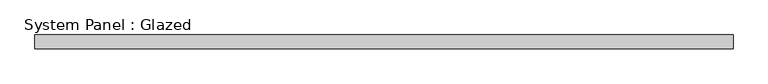
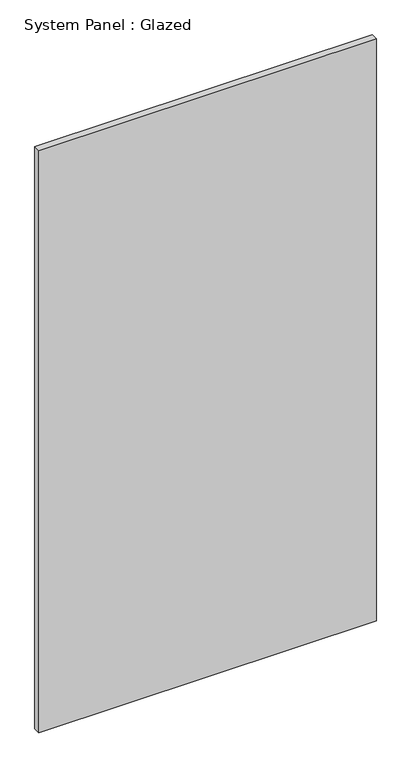
"""IFC4 building model written with IfcOpenShell, lengths in millimetres: plate geometry, System Panel : Glazed."""

from ifc_helpers import new_model, si_unit, origin, origin_with_axes, place, context, project, spatial, polyline, outline, extrude, source, transform, mapped, element, save


def system_panel_glazed_23a28a9f(model_context):
    return source(origin(), model_context, "Body", "SweptSolid", [
        extrude(outline(polyline([(651.4041668, 19.05), (-651.4041668, 19.05), (-651.4041668, 44.45), (651.4041668, 44.45), (651.4041668, 19.05)])), origin_with_axes(), (0.0, 0.0, 1.0), 2374.9),
    ])


if __name__ == "__main__":
    model = new_model("IFC4")
    model_context = context("Model", 3, world=origin())
    ifc_project = project(units=[si_unit("LENGTHUNIT", "METRE", prefix="MILLI")], contexts=[model_context])
    site = spatial("IfcSite", under=ifc_project)
    building = spatial("IfcBuilding", under=site)
    placement = place(None, origin())
    system_panel_glazed_shape = system_panel_glazed_23a28a9f(model_context)
    element("IfcPlate", 1, ObjectType="System Panel : Glazed", at=placement, inside=building, context=model_context, shape_type="MappedRepresentation", body=[
        mapped(system_panel_glazed_shape, transform((0.0, 0.0, 0.0), x_axis=(1.0, 0.0, 0.0), y_axis=(0.0, 1.0, 0.0), z_axis=(0.0, 0.0, 1.0))),
    ])
    save(model, "model.ifc")

# Revit data of these elements
# Type "System Panel : Glazed"
#   Construction Type Id = "GSP4R"
#   Analytic Construction = "1/8 in Pilkington single glazing"
#   Visual Light Transmittance = 0.9
#   Solar Heat Gain Coefficient = 0.86
#   Heat Transfer Coefficient (U) = 1.18115 BTU/(h·ft²·°F)
#   Define Thermal Properties by = 1
# Element 1 (IfcPlate, "System Panel : Glazed")
#   Materials on its faces: "Glass"
# Materials
#   "Glass": class "Glass", colour RGB 0 128 192, transparency 0.75, Description = "Soda Lime Glass", Cost = 0
